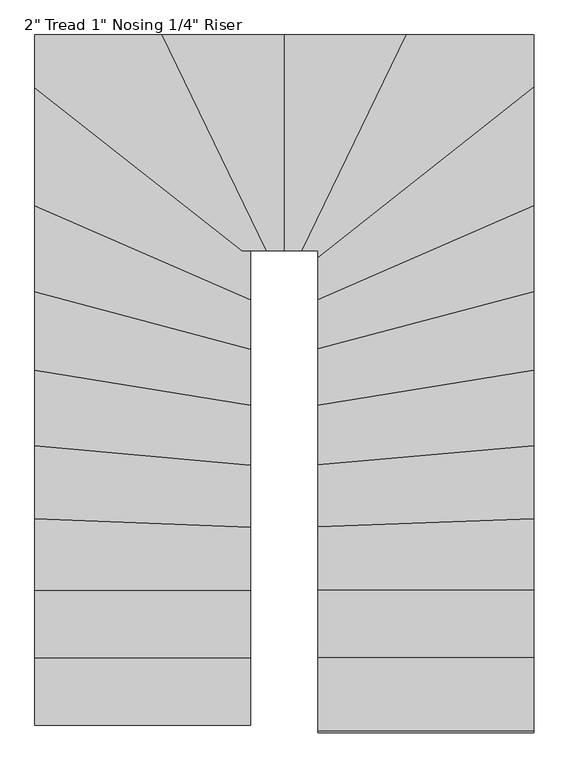
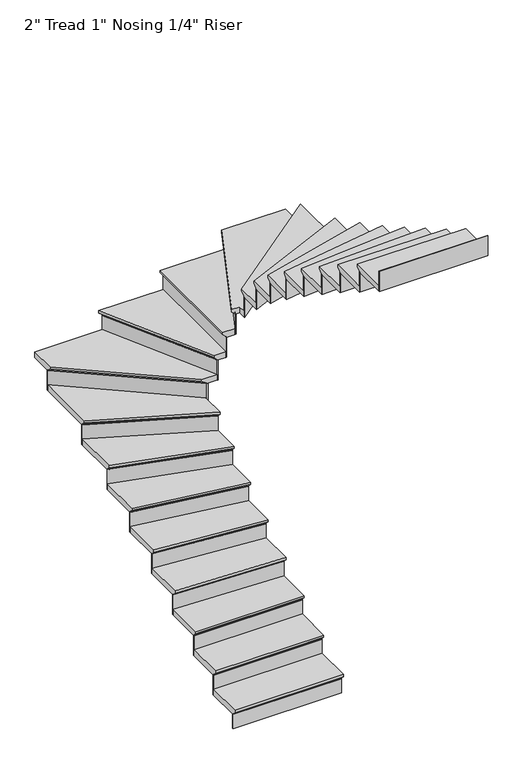
"""IFC4 building model written with IfcOpenShell, lengths in millimetres: stair flight geometry."""

from ifc_helpers import new_model, si_unit, origin, place, context, project, spatial, faceted_brep, source, transform, mapped, element, save


def stair_flight_777e5497(model_context):
    return source(origin(), model_context, "Body", "Brep", [
        faceted_brep([(-5047.1987704, -4554.2130548, 11127.9214286), (-5047.1987704, -4554.2130548, 11146.9714286), (-5940.8822214, -4554.2130548, 11146.9714286), (-5940.8822214, -4554.2130548, 11127.9214286), (-5047.1987704, -4528.8130548, 11102.5214286), (-5940.8822214, -4528.8130548, 11102.5214286), (-5047.1987704, -4249.4130548, 11146.9714286), (-5940.8822214, -4249.4130548, 11146.9714286), (-5940.8822214, -4528.8130548, 11096.1714286), (-5940.8822214, -4249.4130548, 11096.1714286), (-5047.1987704, -4249.4130548, 11096.1714286), (-5047.1987704, -4528.8130548, 11096.1714286)], [[[0, 1, 2, 3]], [[4, 0, 3, 5]], [[2, 1, 6, 7]], [[8, 9, 10, 11]], [[2, 7, 9, 8, 5, 3]], [[8, 11, 4, 5]], [[6, 1, 0, 4, 11, 10]], [[7, 6, 10, 9]]]),
        faceted_brep([(-5047.1987704, -4528.8130548, 11096.1714286), (-5047.1987704, -4528.8130548, 10972.8), (-5047.1987704, -4522.4630548, 10972.8), (-5047.1987704, -4522.4630548, 11096.1714286), (-5940.8822214, -4528.8130548, 11096.1714286), (-5940.8822214, -4522.4630548, 11096.1714286), (-5940.8822214, -4522.4630548, 10972.8), (-5940.8822214, -4528.8130548, 10972.8)], [[[0, 1, 2, 3]], [[4, 5, 6, 7]], [[1, 0, 4, 7]], [[2, 1, 7, 6]], [[3, 2, 6, 5]], [[0, 3, 5, 4]]]),
        faceted_brep([(-5047.1987704, -4249.4130548, 11270.3428571), (-5047.1987704, -4249.4130548, 11096.1714286), (-5047.1987704, -4243.0630548, 11096.1714286), (-5047.1987704, -4243.0630548, 11270.3428571), (-5940.8822214, -4249.4130548, 11270.3428571), (-5940.8822214, -4243.0630548, 11270.3428571), (-5940.8822214, -4243.0630548, 11096.1714286), (-5940.8822214, -4249.4130548, 11096.1714286)], [[[0, 1, 2, 3]], [[4, 5, 6, 7]], [[1, 0, 4, 7]], [[2, 1, 7, 6]], [[3, 2, 6, 5]], [[0, 3, 5, 4]]]),
        faceted_brep([(-5940.8822214, -4274.8130548, 11321.1428571), (-5047.1987704, -4274.8130548, 11321.1428571), (-5047.1987704, -3970.0130548, 11321.1428571), (-5940.8822214, -3970.0130548, 11321.1428571), (-5940.8822214, -4249.4130548, 11270.3428571), (-5940.8822214, -3970.0130548, 11270.3428571), (-5047.1987704, -3970.0130548, 11270.3428571), (-5047.1987704, -4249.4130548, 11270.3428571), (-5940.8822214, -4249.4130548, 11276.6928571), (-5940.8822214, -4274.8130548, 11302.0928571), (-5047.1987704, -4249.4130548, 11276.6928571), (-5047.1987704, -4274.8130548, 11302.0928571)], [[[0, 1, 2, 3]], [[4, 5, 6, 7]], [[0, 3, 5, 4, 8, 9]], [[4, 7, 10, 8]], [[2, 1, 11, 10, 7, 6]], [[3, 2, 6, 5]], [[11, 1, 0, 9]], [[10, 11, 9, 8]]]),
        faceted_brep([(-5047.1987704, -3970.0130548, 11444.5142857), (-5047.1987704, -3970.0130548, 11270.3428571), (-5047.1987704, -3963.6630548, 11270.3428571), (-5047.1987704, -3963.6630548, 11444.5142857), (-5940.8822214, -3970.0130548, 11444.5142857), (-5940.8822214, -3963.6630548, 11444.5142857), (-5940.8822214, -3963.6630548, 11270.3428571), (-5940.8822214, -3970.0130548, 11270.3428571)], [[[0, 1, 2, 3]], [[4, 5, 6, 7]], [[1, 0, 4, 7]], [[2, 1, 7, 6]], [[3, 2, 6, 5]], [[0, 3, 5, 4]]]),
        faceted_brep([(-5940.8822214, -3995.4130548, 11495.3142857), (-5047.1987704, -3995.4130548, 11495.3142857), (-5047.1987704, -3707.9036879, 11495.3142857), (-5940.8822214, -3673.2843203, 11495.3142857), (-5940.8822214, -3970.0130548, 11444.5142857), (-5940.8822214, -3673.2843203, 11444.5142857), (-5047.1987704, -3707.9036879, 11444.5142857), (-5047.1987704, -3970.0130548, 11444.5142857), (-5940.8822214, -3970.0130548, 11450.8642857), (-5940.8822214, -3995.4130548, 11476.2642857), (-5047.1987704, -3970.0130548, 11450.8642857), (-5047.1987704, -3995.4130548, 11476.2642857)], [[[0, 1, 2, 3]], [[4, 5, 6, 7]], [[0, 3, 5, 4, 8, 9]], [[4, 7, 10, 8]], [[2, 1, 11, 10, 7, 6]], [[3, 2, 6, 5]], [[11, 1, 0, 9]], [[10, 11, 9, 8]]]),
        faceted_brep([(-5047.1987704, -3707.9036879, 11618.6857143), (-5047.1987704, -3707.9036879, 11444.5142857), (-5047.1987704, -3701.5489252, 11444.5142857), (-5047.1987704, -3701.5489252, 11618.6857143), (-5940.8822214, -3673.2843203, 11618.6857143), (-5940.8822214, -3666.9295576, 11618.6857143), (-5940.8822214, -3666.9295576, 11444.5142857), (-5940.8822214, -3673.2843203, 11444.5142857)], [[[0, 1, 2, 3]], [[4, 5, 6, 7]], [[1, 0, 4, 7]], [[2, 1, 7, 6]], [[3, 2, 6, 5]], [[0, 3, 5, 4]]]),
        faceted_brep([(-5940.8822214, -3698.703371, 11669.4857143), (-5047.1987704, -3733.3227386, 11669.4857143), (-5047.1987704, -3451.3234819, 11669.4857143), (-5940.8822214, -3370.89733, 11669.4857143), (-5940.8822214, -3673.2843203, 11618.6857143), (-5940.8822214, -3370.89733, 11618.6857143), (-5047.1987704, -3451.3234819, 11618.6857143), (-5047.1987704, -3707.9036879, 11618.6857143), (-5940.8822214, -3673.2843203, 11625.0357143), (-5940.8822214, -3698.703371, 11650.4357143), (-5047.1987704, -3707.9036879, 11625.0357143), (-5047.1987704, -3733.3227386, 11650.4357143)], [[[0, 1, 2, 3]], [[4, 5, 6, 7]], [[0, 3, 5, 4, 8, 9]], [[4, 7, 10, 8]], [[2, 1, 11, 10, 7, 6]], [[3, 2, 6, 5]], [[11, 1, 0, 9]], [[10, 11, 9, 8]]]),
        faceted_brep([(-5047.1987704, -3451.3234819, 11792.8571429), (-5047.1987704, -3451.3234819, 11618.6857143), (-5047.1987704, -3444.9478197, 11618.6857143), (-5047.1987704, -3444.9478197, 11792.8571429), (-5940.8822214, -3370.89733, 11792.8571429), (-5940.8822214, -3364.5216678, 11792.8571429), (-5940.8822214, -3364.5216678, 11618.6857143), (-5940.8822214, -3370.89733, 11618.6857143)], [[[0, 1, 2, 3]], [[4, 5, 6, 7]], [[1, 0, 4, 7]], [[2, 1, 7, 6]], [[3, 2, 6, 5]], [[0, 3, 5, 4]]]),
        faceted_brep([(-5940.8822214, -3396.3999789, 11843.6571429), (-5047.1987704, -3476.8261308, 11843.6571429), (-5047.1987704, -3203.4301079, 11843.6571429), (-5940.8822214, -3059.5417727, 11843.6571429), (-5940.8822214, -3370.89733, 11792.8571429), (-5940.8822214, -3059.5417727, 11792.8571429), (-5047.1987704, -3203.4301079, 11792.8571429), (-5047.1987704, -3451.3234819, 11792.8571429), (-5940.8822214, -3370.89733, 11799.2071429), (-5940.8822214, -3396.3999789, 11824.6071429), (-5047.1987704, -3451.3234819, 11799.2071429), (-5047.1987704, -3476.8261308, 11824.6071429)], [[[0, 1, 2, 3]], [[4, 5, 6, 7]], [[0, 3, 5, 4, 8, 9]], [[4, 7, 10, 8]], [[2, 1, 11, 10, 7, 6]], [[3, 2, 6, 5]], [[11, 1, 0, 9]], [[10, 11, 9, 8]]]),
        faceted_brep([(-5047.1987704, -3203.4301079, 11967.0285714), (-5047.1987704, -3203.4301079, 11792.8571429), (-5047.1987704, -3196.9983292, 11792.8571429), (-5047.1987704, -3196.9983292, 11967.0285714), (-5940.8822214, -3059.5417727, 11967.0285714), (-5940.8822214, -3053.109994, 11967.0285714), (-5940.8822214, -3053.109994, 11792.8571429), (-5940.8822214, -3059.5417727, 11792.8571429)], [[[0, 1, 2, 3]], [[4, 5, 6, 7]], [[1, 0, 4, 7]], [[2, 1, 7, 6]], [[3, 2, 6, 5]], [[0, 3, 5, 4]]]),
        faceted_brep([(-5940.8822214, -3085.2688872, 12017.8285714), (-5047.1987704, -3229.1572224, 12017.8285714), (-5047.1987704, -2970.3553609, 12017.8285714), (-5940.8822214, -2732.7052783, 12017.8285714), (-5940.8822214, -3059.5417727, 11967.0285714), (-5940.8822214, -2732.7052783, 11967.0285714), (-5047.1987704, -2970.3553609, 11967.0285714), (-5047.1987704, -3203.4301079, 11967.0285714), (-5940.8822214, -3059.5417727, 11973.3785714), (-5940.8822214, -3085.2688872, 11998.7785714), (-5047.1987704, -3203.4301079, 11973.3785714), (-5047.1987704, -3229.1572224, 11998.7785714)], [[[0, 1, 2, 3]], [[4, 5, 6, 7]], [[0, 3, 5, 4, 8, 9]], [[4, 7, 10, 8]], [[2, 1, 11, 10, 7, 6]], [[3, 2, 6, 5]], [[11, 1, 0, 9]], [[10, 11, 9, 8]]]),
        faceted_brep([(-5047.1987704, -2970.3553609, 12141.2), (-5047.1987704, -2970.3553609, 11967.0285714), (-5047.1987704, -2963.7846771, 11967.0285714), (-5047.1987704, -2963.7846771, 12141.2), (-5940.8822214, -2732.7052783, 12141.2), (-5940.8822214, -2726.1345945, 12141.2), (-5940.8822214, -2726.1345945, 11967.0285714), (-5940.8822214, -2732.7052783, 11967.0285714)], [[[0, 1, 2, 3]], [[4, 5, 6, 7]], [[1, 0, 4, 7]], [[2, 1, 7, 6]], [[3, 2, 6, 5]], [[0, 3, 5, 4]]]),
        faceted_brep([(-5940.8822214, -2758.9880136, 12192.0), (-5047.1987704, -2996.6380961, 12192.0), (-5047.1987704, -2765.8050203, 12192.0), (-5940.8822214, -2375.5896532, 12192.0), (-5940.8822214, -2732.7052783, 12141.2), (-5940.8822214, -2375.5896532, 12141.2), (-5047.1987704, -2765.8050203, 12141.2), (-5047.1987704, -2970.3553609, 12141.2), (-5940.8822214, -2732.7052783, 12147.55), (-5940.8822214, -2758.9880136, 12172.95), (-5047.1987704, -2970.3553609, 12147.55), (-5047.1987704, -2996.6380961, 12172.95)], [[[0, 1, 2, 3]], [[4, 5, 6, 7]], [[0, 3, 5, 4, 8, 9]], [[4, 7, 10, 8]], [[2, 1, 11, 10, 7, 6]], [[3, 2, 6, 5]], [[11, 1, 0, 9]], [[10, 11, 9, 8]]]),
        faceted_brep([(-5047.1987704, -2765.8050203, 12315.3714286), (-5047.1987704, -2765.8050203, 12141.2), (-5047.1987704, -2758.8760908, 12141.2), (-5047.1987704, -2758.8760908, 12315.3714286), (-5940.8822214, -2375.5896532, 12315.3714286), (-5940.8822214, -2368.6607237, 12315.3714286), (-5940.8822214, -2368.6607237, 12141.2), (-5940.8822214, -2375.5896532, 12141.2)], [[[0, 1, 2, 3]], [[4, 5, 6, 7]], [[1, 0, 4, 7]], [[2, 1, 7, 6]], [[3, 2, 6, 5]], [[0, 3, 5, 4]]]),
        faceted_brep([(-5940.8822214, -2403.3053713, 12366.1714286), (-5047.1987704, -2793.5207384, 12366.1714286), (-5047.1987704, -2590.8424524, 12366.1714286), (-5040.8038639, -2590.8424524, 12366.1714286), (-5940.8822214, -1882.1944717, 12366.1714286), (-5940.8822214, -2375.5896532, 12315.3714286), (-5940.8822214, -1882.1944717, 12315.3714286), (-5040.8038639, -2590.8424524, 12315.3714286), (-5047.1987704, -2590.8424524, 12315.3714286), (-5047.1987704, -2765.8050203, 12315.3714286), (-5940.8822214, -2375.5896532, 12321.7214286), (-5940.8822214, -2403.3053713, 12347.1214286), (-5047.1987704, -2765.8050203, 12321.7214286), (-5047.1987704, -2793.5207384, 12347.1214286)], [[[0, 1, 2, 3, 4]], [[5, 6, 7, 8, 9]], [[0, 4, 6, 5, 10, 11]], [[5, 9, 12, 10]], [[2, 1, 13, 12, 9, 8]], [[4, 3, 7, 6]], [[13, 1, 0, 11]], [[12, 13, 11, 10]], [[3, 2, 8, 7]]]),
        faceted_brep([(-5040.8038639, -2590.8424524, 12489.5428571), (-5040.8038639, -2590.8424524, 12315.3714286), (-5030.5387554, -2590.8424524, 12315.3714286), (-5030.5387554, -2590.8424524, 12489.5428571), (-5940.8822214, -1882.1944717, 12489.5428571), (-5940.8822214, -1874.1125661, 12489.5428571), (-5940.8822214, -1874.1125661, 12315.3714286), (-5940.8822214, -1882.1944717, 12315.3714286)], [[[0, 1, 2, 3]], [[4, 5, 6, 7]], [[1, 0, 4, 7]], [[2, 1, 7, 6]], [[3, 2, 6, 5]], [[0, 3, 5, 4]]]),
        faceted_brep([(-5384.6489457, -1697.1590014, 12540.3428571), (-5940.8822214, -1697.1590014, 12540.3428571), (-5940.8822214, -1914.5220945, 12540.3428571), (-5081.8642978, -2590.8424524, 12540.3428571), (-4952.3566185, -2590.8424524, 12540.3428571), (-5940.8822214, -1697.1590014, 12489.5428571), (-5384.6489457, -1697.1590014, 12489.5428571), (-4952.3566185, -2590.8424524, 12489.5428571), (-5040.8038639, -2590.8424524, 12489.5428571), (-5940.8822214, -1882.1944717, 12489.5428571), (-5940.8822214, -1882.1944717, 12495.8928571), (-5940.8822214, -1914.5220945, 12521.2928571), (-5040.8038639, -2590.8424524, 12495.8928571), (-5081.8642978, -2590.8424524, 12521.2928571)], [[[0, 1, 2, 3, 4]], [[5, 6, 7, 8, 9]], [[1, 0, 6, 5]], [[2, 1, 5, 9, 10, 11]], [[9, 8, 12, 10]], [[4, 3, 13, 12, 8, 7]], [[0, 4, 7, 6]], [[13, 3, 2, 11]], [[12, 13, 11, 10]]]),
        faceted_brep([(-4952.3566185, -2590.8424524, 12663.7142857), (-4952.3566185, -2590.8424524, 12489.5428571), (-4945.3027294, -2590.8424524, 12489.5428571), (-4945.3027294, -2590.8424524, 12663.7142857), (-5384.6489457, -1697.1590014, 12663.7142857), (-5377.5950566, -1697.1590014, 12663.7142857), (-5377.5950566, -1697.1590014, 12489.5428571), (-5384.6489457, -1697.1590014, 12489.5428571)], [[[0, 1, 2, 3]], [[4, 5, 6, 7]], [[1, 0, 4, 7]], [[2, 1, 7, 6]], [[3, 2, 6, 5]], [[0, 3, 5, 4]]]),
        faceted_brep([(-5412.8645022, -1697.1590014, 12714.5142857), (-4980.5721749, -2590.8424524, 12714.5142857), (-4882.0987704, -2590.8424524, 12714.5142857), (-4882.0987706, -1697.1590014, 12714.5142857), (-5384.6489457, -1697.1590014, 12663.7142857), (-4882.0987706, -1697.1590014, 12663.7142857), (-4882.0987704, -2590.8424524, 12663.7142857), (-4952.3566185, -2590.8424524, 12663.7142857), (-5384.6489457, -1697.1590014, 12670.0642857), (-5412.8645022, -1697.1590014, 12695.4642857), (-4952.3566185, -2590.8424524, 12670.0642857), (-4980.5721749, -2590.8424524, 12695.4642857)], [[[0, 1, 2, 3]], [[4, 5, 6, 7]], [[0, 3, 5, 4, 8, 9]], [[4, 7, 10, 8]], [[3, 2, 6, 5]], [[11, 1, 0, 9]], [[10, 11, 9, 8]], [[2, 1, 11, 10, 7, 6]]]),
        faceted_brep([(-4882.0987704, -2590.8424524, 12837.8857143), (-4882.0987704, -2590.8424524, 12663.7142857), (-4875.7487704, -2590.8424524, 12663.7142857), (-4875.7487704, -2590.8424524, 12837.8857143), (-4882.0987706, -1697.1590014, 12837.8857143), (-4875.7487706, -1697.1590014, 12837.8857143), (-4875.7487706, -1697.1590014, 12663.7142857), (-4882.0987706, -1697.1590014, 12663.7142857)], [[[0, 1, 2, 3]], [[4, 5, 6, 7]], [[1, 0, 4, 7]], [[2, 1, 7, 6]], [[3, 2, 6, 5]], [[0, 3, 5, 4]]]),
        faceted_brep([(-4907.4987706, -1697.1590014, 12888.6857143), (-4907.4987704, -2590.8424524, 12888.6857143), (-4806.2098095, -2590.8424524, 12888.6857143), (-4373.9174828, -1697.1590014, 12888.6857143), (-4882.0987706, -1697.1590014, 12837.8857143), (-4373.9174828, -1697.1590014, 12837.8857143), (-4806.2098095, -2590.8424524, 12837.8857143), (-4882.0987704, -2590.8424524, 12837.8857143), (-4882.0987706, -1697.1590014, 12844.2357143), (-4907.4987706, -1697.1590014, 12869.6357143), (-4882.0987704, -2590.8424524, 12844.2357143), (-4907.4987704, -2590.8424524, 12869.6357143)], [[[0, 1, 2, 3]], [[4, 5, 6, 7]], [[0, 3, 5, 4, 8, 9]], [[4, 7, 10, 8]], [[2, 1, 11, 10, 7, 6]], [[3, 2, 6, 5]], [[11, 1, 0, 9]], [[10, 11, 9, 8]]]),
        faceted_brep([(-4806.2098095, -2590.8424524, 13012.0571429), (-4806.2098095, -2590.8424524, 12837.8857143), (-4799.1559204, -2590.8424524, 12837.8857143), (-4799.1559204, -2590.8424524, 13012.0571429), (-4373.9174828, -1697.1590014, 13012.0571429), (-4366.8635937, -1697.1590014, 13012.0571429), (-4366.8635937, -1697.1590014, 12837.8857143), (-4373.9174828, -1697.1590014, 12837.8857143)], [[[0, 1, 2, 3]], [[4, 5, 6, 7]], [[1, 0, 4, 7]], [[2, 1, 7, 6]], [[3, 2, 6, 5]], [[0, 3, 5, 4]]]),
        faceted_brep([(-3874.1153195, -1946.8497166, 13062.8571429), (-3874.1153195, -1697.1590014, 13062.8571429), (-4402.1330392, -1697.1590014, 13062.8571429), (-4834.4253659, -2590.8424524, 13062.8571429), (-4767.7987704, -2590.8424524, 13062.8571429), (-4767.7987704, -2650.4628721, 13062.8571429), (-3874.1153195, -1697.1590014, 13012.0571429), (-3874.1153195, -1946.8497166, 13012.0571429), (-4767.7987704, -2650.4628721, 13012.0571429), (-4767.7987704, -2590.8424524, 13012.0571429), (-4806.2098095, -2590.8424524, 13012.0571429), (-4373.9174828, -1697.1590014, 13012.0571429), (-4806.2098095, -2590.8424524, 13018.4071429), (-4373.9174828, -1697.1590014, 13018.4071429), (-4834.4253659, -2590.8424524, 13043.8071429), (-4402.1330392, -1697.1590014, 13043.8071429)], [[[0, 1, 2, 3, 4, 5]], [[6, 7, 8, 9, 10, 11]], [[1, 0, 7, 6]], [[11, 10, 12, 13]], [[4, 3, 14, 12, 10, 9]], [[5, 4, 9, 8]], [[0, 5, 8, 7]], [[14, 3, 2, 15]], [[12, 14, 15, 13]], [[2, 1, 6, 11, 13, 15]]]),
        faceted_brep([(-4767.7987704, -2650.4628721, 13186.2285714), (-4767.7987704, -2650.4628721, 13012.0571429), (-4767.7987704, -2658.5447778, 13012.0571429), (-4767.7987704, -2658.5447778, 13186.2285714), (-3874.1153195, -1946.8497166, 13186.2285714), (-3874.1153195, -1954.9316222, 13186.2285714), (-3874.1153195, -1954.9316222, 13012.0571429), (-3874.1153195, -1946.8497166, 13012.0571429)], [[[0, 1, 2, 3]], [[4, 5, 6, 7]], [[1, 0, 4, 7]], [[2, 1, 7, 6]], [[3, 2, 6, 5]], [[0, 3, 5, 4]]]),
        faceted_brep([(-3874.1153195, -1914.5220938, 13237.0285714), (-4767.7987704, -2618.1352494, 13237.0285714), (-4767.7987704, -2821.2364563, 13237.0285714), (-3874.1153195, -2431.0210889, 13237.0285714), (-3874.1153195, -1946.8497166, 13186.2285714), (-3874.1153195, -2431.0210889, 13186.2285714), (-4767.7987704, -2821.2364563, 13186.2285714), (-4767.7987704, -2650.4628721, 13186.2285714), (-3874.1153195, -1946.8497166, 13192.5785714), (-3874.1153195, -1914.5220938, 13217.9785714), (-4767.7987704, -2650.4628721, 13192.5785714), (-4767.7987704, -2618.1352494, 13217.9785714)], [[[0, 1, 2, 3]], [[4, 5, 6, 7]], [[0, 3, 5, 4, 8, 9]], [[4, 7, 10, 8]], [[2, 1, 11, 10, 7, 6]], [[3, 2, 6, 5]], [[11, 1, 0, 9]], [[10, 11, 9, 8]]]),
        faceted_brep([(-4767.7987704, -2821.2364563, 13360.4), (-4767.7987704, -2821.2364563, 13186.2285714), (-4767.7987704, -2828.1653858, 13186.2285714), (-4767.7987704, -2828.1653858, 13360.4), (-3874.1153195, -2431.0210889, 13360.4), (-3874.1153195, -2437.9500185, 13360.4), (-3874.1153195, -2437.9500185, 13186.2285714), (-3874.1153195, -2431.0210889, 13186.2285714)], [[[0, 1, 2, 3]], [[4, 5, 6, 7]], [[1, 0, 4, 7]], [[2, 1, 7, 6]], [[3, 2, 6, 5]], [[0, 3, 5, 4]]]),
        faceted_brep([(-3874.1153195, -2403.3053709, 13411.2), (-4767.7987704, -2793.5207382, 13411.2), (-4767.7987704, -3022.9208311, 13411.2), (-3874.1153195, -2785.2707484, 13411.2), (-3874.1153195, -2431.0210889, 13360.4), (-3874.1153195, -2785.2707484, 13360.4), (-4767.7987704, -3022.9208311, 13360.4), (-4767.7987704, -2821.2364563, 13360.4), (-3874.1153195, -2431.0210889, 13366.75), (-3874.1153195, -2403.3053709, 13392.15), (-4767.7987704, -2821.2364563, 13366.75), (-4767.7987704, -2793.5207382, 13392.15)], [[[0, 1, 2, 3]], [[4, 5, 6, 7]], [[0, 3, 5, 4, 8, 9]], [[4, 7, 10, 8]], [[2, 1, 11, 10, 7, 6]], [[3, 2, 6, 5]], [[11, 1, 0, 9]], [[10, 11, 9, 8]]]),
        faceted_brep([(-4767.7987704, -3022.9208311, 13534.5714286), (-4767.7987704, -3022.9208311, 13360.4), (-4767.7987704, -3029.4915149, 13360.4), (-4767.7987704, -3029.4915149, 13534.5714286), (-3874.1153195, -2785.2707484, 13534.5714286), (-3874.1153195, -2791.8414322, 13534.5714286), (-3874.1153195, -2791.8414322, 13360.4), (-3874.1153195, -2785.2707484, 13360.4)], [[[0, 1, 2, 3]], [[4, 5, 6, 7]], [[1, 0, 4, 7]], [[2, 1, 7, 6]], [[3, 2, 6, 5]], [[0, 3, 5, 4]]]),
        faceted_brep([(-3874.1153195, -2758.9880132, 13585.3714286), (-4767.7987704, -2996.6380959, 13585.3714286), (-4767.7987704, -3254.8843368, 13585.3714286), (-3874.1153195, -3110.9960015, 13585.3714286), (-3874.1153195, -2785.2707484, 13534.5714286), (-3874.1153195, -3110.9960015, 13534.5714286), (-4767.7987704, -3254.8843368, 13534.5714286), (-4767.7987704, -3022.9208311, 13534.5714286), (-3874.1153195, -2785.2707484, 13540.9214286), (-3874.1153195, -2758.9880132, 13566.3214286), (-4767.7987704, -3022.9208311, 13540.9214286), (-4767.7987704, -2996.6380959, 13566.3214286)], [[[0, 1, 2, 3]], [[4, 5, 6, 7]], [[0, 3, 5, 4, 8, 9]], [[4, 7, 10, 8]], [[2, 1, 11, 10, 7, 6]], [[3, 2, 6, 5]], [[11, 1, 0, 9]], [[10, 11, 9, 8]]]),
        faceted_brep([(-4767.7987704, -3254.8843368, 13708.7428571), (-4767.7987704, -3254.8843368, 13534.5714286), (-4767.7987704, -3261.3161154, 13534.5714286), (-4767.7987704, -3261.3161154, 13708.7428571), (-3874.1153195, -3110.9960015, 13708.7428571), (-3874.1153195, -3117.4277801, 13708.7428571), (-3874.1153195, -3117.4277801, 13534.5714286), (-3874.1153195, -3110.9960015, 13534.5714286)], [[[0, 1, 2, 3]], [[4, 5, 6, 7]], [[1, 0, 4, 7]], [[2, 1, 7, 6]], [[3, 2, 6, 5]], [[0, 3, 5, 4]]]),
        faceted_brep([(-3874.1153195, -3085.2688869, 13759.5428571), (-4767.7987704, -3229.1572222, 13759.5428571), (-4767.7987704, -3502.3287795, 13759.5428571), (-3874.1153195, -3421.9026274, 13759.5428571), (-3874.1153195, -3110.9960015, 13708.7428571), (-3874.1153195, -3421.9026274, 13708.7428571), (-4767.7987704, -3502.3287795, 13708.7428571), (-4767.7987704, -3254.8843368, 13708.7428571), (-3874.1153195, -3110.9960015, 13715.0928571), (-3874.1153195, -3085.2688869, 13740.4928571), (-4767.7987704, -3254.8843368, 13715.0928571), (-4767.7987704, -3229.1572222, 13740.4928571)], [[[0, 1, 2, 3]], [[4, 5, 6, 7]], [[0, 3, 5, 4, 8, 9]], [[4, 7, 10, 8]], [[2, 1, 11, 10, 7, 6]], [[3, 2, 6, 5]], [[11, 1, 0, 9]], [[10, 11, 9, 8]]]),
        faceted_brep([(-4767.7987704, -3502.3287795, 13882.9142857), (-4767.7987704, -3502.3287795, 13708.7428571), (-4767.7987704, -3508.7044417, 13708.7428571), (-4767.7987704, -3508.7044417, 13882.9142857), (-3874.1153195, -3421.9026274, 13882.9142857), (-3874.1153195, -3428.2782897, 13882.9142857), (-3874.1153195, -3428.2782897, 13708.7428571), (-3874.1153195, -3421.9026274, 13708.7428571)], [[[0, 1, 2, 3]], [[4, 5, 6, 7]], [[1, 0, 4, 7]], [[2, 1, 7, 6]], [[3, 2, 6, 5]], [[0, 3, 5, 4]]]),
        faceted_brep([(-3874.1153195, -3396.3999786, 13933.7142857), (-4767.7987704, -3476.8261306, 13933.7142857), (-4767.7987704, -3758.7417891, 13933.7142857), (-3874.1153195, -3724.1224215, 13933.7142857), (-3874.1153195, -3421.9026274, 13882.9142857), (-3874.1153195, -3724.1224215, 13882.9142857), (-4767.7987704, -3758.7417891, 13882.9142857), (-4767.7987704, -3502.3287795, 13882.9142857), (-3874.1153195, -3421.9026274, 13889.2642857), (-3874.1153195, -3396.3999786, 13914.6642857), (-4767.7987704, -3502.3287795, 13889.2642857), (-4767.7987704, -3476.8261306, 13914.6642857)], [[[0, 1, 2, 3]], [[4, 5, 6, 7]], [[0, 3, 5, 4, 8, 9]], [[4, 7, 10, 8]], [[2, 1, 11, 10, 7, 6]], [[3, 2, 6, 5]], [[11, 1, 0, 9]], [[10, 11, 9, 8]]]),
        faceted_brep([(-4767.7987704, -3758.7417891, 14057.0857143), (-4767.7987704, -3758.7417891, 13882.9142857), (-4767.7987704, -3765.0965518, 13882.9142857), (-4767.7987704, -3765.0965518, 14057.0857143), (-3874.1153195, -3724.1224215, 14057.0857143), (-3874.1153195, -3730.4771842, 14057.0857143), (-3874.1153195, -3730.4771842, 13882.9142857), (-3874.1153195, -3724.1224215, 13882.9142857)], [[[0, 1, 2, 3]], [[4, 5, 6, 7]], [[1, 0, 4, 7]], [[2, 1, 7, 6]], [[3, 2, 6, 5]], [[0, 3, 5, 4]]]),
        faceted_brep([(-3874.1153195, -3698.7033708, 14107.8857143), (-4767.7987704, -3733.3227384, 14107.8857143), (-4767.7987704, -4020.8130546, 14107.8857143), (-3874.1153195, -4020.8130546, 14107.8857143), (-3874.1153195, -3724.1224215, 14057.0857143), (-3874.1153195, -4020.8130546, 14057.0857143), (-4767.7987704, -4020.8130546, 14057.0857143), (-4767.7987704, -3758.7417891, 14057.0857143), (-3874.1153195, -3724.1224215, 14063.4357143), (-3874.1153195, -3698.7033708, 14088.8357143), (-4767.7987704, -3758.7417891, 14063.4357143), (-4767.7987704, -3733.3227384, 14088.8357143)], [[[0, 1, 2, 3]], [[4, 5, 6, 7]], [[0, 3, 5, 4, 8, 9]], [[4, 7, 10, 8]], [[2, 1, 11, 10, 7, 6]], [[3, 2, 6, 5]], [[11, 1, 0, 9]], [[10, 11, 9, 8]]]),
        faceted_brep([(-4767.7987704, -4020.8130546, 14231.2571429), (-4767.7987704, -4020.8130546, 14057.0857143), (-4767.7987704, -4027.1630546, 14057.0857143), (-4767.7987704, -4027.1630546, 14231.2571429), (-3874.1153195, -4020.8130546, 14231.2571429), (-3874.1153195, -4027.1630546, 14231.2571429), (-3874.1153195, -4027.1630546, 14057.0857143), (-3874.1153195, -4020.8130546, 14057.0857143)], [[[0, 1, 2, 3]], [[4, 5, 6, 7]], [[1, 0, 4, 7]], [[2, 1, 7, 6]], [[3, 2, 6, 5]], [[0, 3, 5, 4]]]),
        faceted_brep([(-3874.1153195, -3995.4130546, 14282.0571429), (-4767.7987704, -3995.4130546, 14282.0571429), (-4767.7987704, -4300.2130546, 14282.0571429), (-3874.1153195, -4300.2130546, 14282.0571429), (-3874.1153195, -4020.8130546, 14231.2571429), (-3874.1153195, -4300.2130546, 14231.2571429), (-4767.7987704, -4300.2130546, 14231.2571429), (-4767.7987704, -4020.8130546, 14231.2571429), (-3874.1153195, -4020.8130546, 14237.6071429), (-3874.1153195, -3995.4130546, 14263.0071429), (-4767.7987704, -4020.8130546, 14237.6071429), (-4767.7987704, -3995.4130546, 14263.0071429)], [[[0, 1, 2, 3]], [[4, 5, 6, 7]], [[0, 3, 5, 4, 8, 9]], [[4, 7, 10, 8]], [[2, 1, 11, 10, 7, 6]], [[3, 2, 6, 5]], [[11, 1, 0, 9]], [[10, 11, 9, 8]]]),
        faceted_brep([(-4767.7987704, -4300.2130546, 14405.4285714), (-4767.7987704, -4300.2130546, 14231.2571429), (-4767.7987704, -4306.5630546, 14231.2571429), (-4767.7987704, -4306.5630546, 14405.4285714), (-3874.1153195, -4300.2130546, 14405.4285714), (-3874.1153195, -4306.5630546, 14405.4285714), (-3874.1153195, -4306.5630546, 14231.2571429), (-3874.1153195, -4300.2130546, 14231.2571429)], [[[0, 1, 2, 3]], [[4, 5, 6, 7]], [[1, 0, 4, 7]], [[2, 1, 7, 6]], [[3, 2, 6, 5]], [[0, 3, 5, 4]]]),
        faceted_brep([(-4767.7987704, -4579.6130546, 14579.6), (-4767.7987704, -4579.6130546, 14405.4285714), (-4767.7987704, -4585.9630546, 14405.4285714), (-4767.7987704, -4585.9630546, 14579.6), (-3874.1153195, -4579.6130546, 14579.6), (-3874.1153195, -4585.9630546, 14579.6), (-3874.1153195, -4585.9630546, 14405.4285714), (-3874.1153195, -4579.6130546, 14405.4285714)], [[[0, 1, 2, 3]], [[4, 5, 6, 7]], [[1, 0, 4, 7]], [[2, 1, 7, 6]], [[3, 2, 6, 5]], [[0, 3, 5, 4]]]),
        faceted_brep([(-3874.1153195, -4274.8130546, 14456.2285714), (-4767.7987704, -4274.8130546, 14456.2285714), (-4767.7987704, -4579.6130546, 14456.2285714), (-3874.1153195, -4579.6130546, 14456.2285714), (-3874.1153195, -4300.2130546, 14405.4285714), (-3874.1153195, -4579.6130546, 14405.4285714), (-4767.7987704, -4579.6130546, 14405.4285714), (-4767.7987704, -4300.2130546, 14405.4285714), (-3874.1153195, -4300.2130546, 14411.7785714), (-3874.1153195, -4274.8130546, 14437.1785714), (-4767.7987704, -4300.2130546, 14411.7785714), (-4767.7987704, -4274.8130546, 14437.1785714)], [[[0, 1, 2, 3]], [[4, 5, 6, 7]], [[0, 3, 5, 4, 8, 9]], [[4, 7, 10, 8]], [[2, 1, 11, 10, 7, 6]], [[3, 2, 6, 5]], [[11, 1, 0, 9]], [[10, 11, 9, 8]]]),
    ])


if __name__ == "__main__":
    model = new_model("IFC4")
    model_context = context("Model", 3, world=origin())
    ifc_project = project(units=[si_unit("LENGTHUNIT", "METRE", prefix="MILLI")], contexts=[model_context])
    site = spatial("IfcSite", under=ifc_project)
    building = spatial("IfcBuilding", under=site)
    placement = place(None, origin())
    stair_flight_shape = stair_flight_777e5497(model_context)
    element("IfcStairFlight", 1, ObjectType="2\" Tread 1\" Nosing 1/4\" Riser", at=placement, inside=building, context=model_context, shape_type="MappedRepresentation", body=[
        mapped(stair_flight_shape, transform((0.0, 0.0, 0.0), x_axis=(1.0, 0.0, 0.0), y_axis=(0.0, 1.0, 0.0), z_axis=(0.0, 0.0, 1.0))),
    ])
    save(model, "model.ifc")

# Revit data of these elements
# Element 1 (IfcStairFlight, "2\" Tread 1\" Nosing 1/4\" Riser")
#   Materials on its faces: "Tile, Porcelain, 4in"
# Materials
#   "Tile, Porcelain, 4in": class "Generic", colour RGB 89 87 158, transparency 0, Description = "Porcelain tile, 4\", white", Cost = 0
